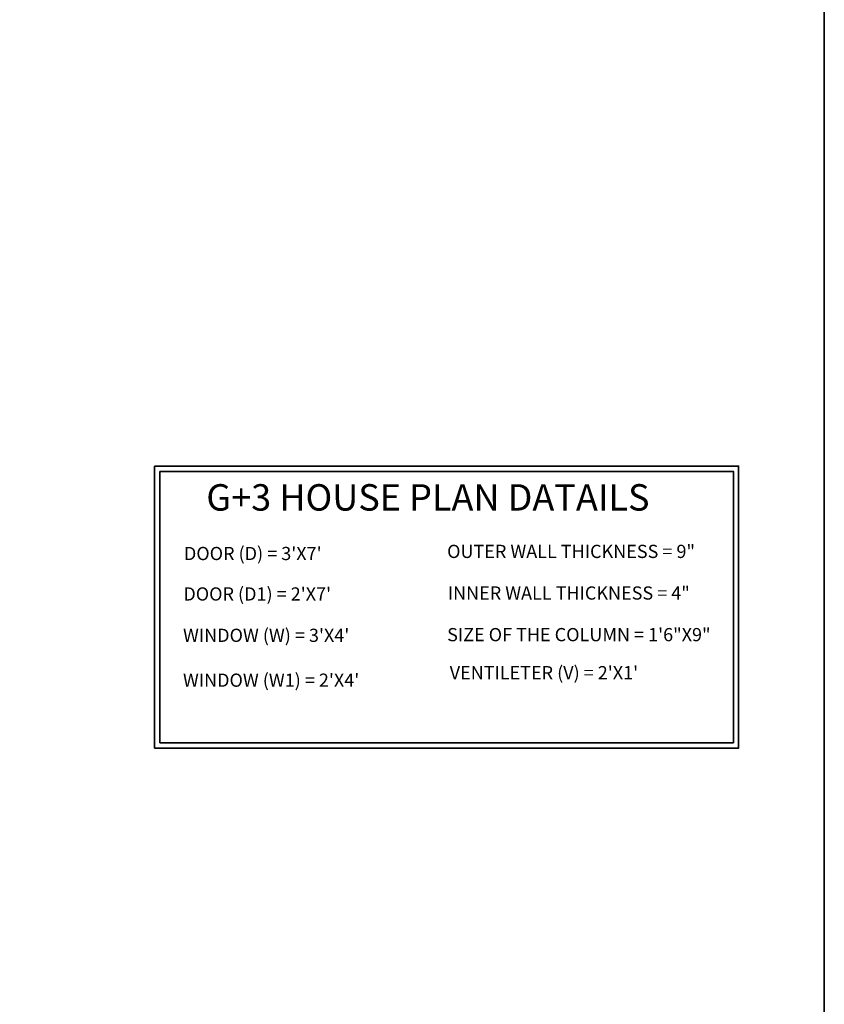
# Model space of a CAD drawing. Units: inches. Extents: x 2391 to 16591, y 7259 to 10239.
# Tile 21 of 27: x 3545 to 4154, y 8500 to 9245. Entities that reach past the tile are written whole.
import ezdxf

# ---------------------------------------------------------------- set-up
doc = ezdxf.new("R2010")
doc.units = ezdxf.units.IN
for name, color, linetype, lineweight in [('A-ANNO-TEXT', 4, 'Continuous', 18), ('A-ANNO-TITL', 3, 'Continuous', 30), ('A-ANNO-TTLB', 7, 'Continuous', 35)]:
    doc.layers.add(name, color=color, linetype=linetype, lineweight=lineweight)
doc.styles.get("Standard").update_dxf_attribs({"font": 'arial.ttf'})

msp = doc.modelspace()

# ---------------------------------------------------------------- linework, layer by layer
at = {"layer": 'A-ANNO-TTLB'}
for points in [[(2391.28, 10239.38), (4154.2, 10239.38), (4154.2, 7258.54), (2391.28, 7258.54)], [(3647.57, 8907.13), (4089.39, 8907.13), (4089.39, 8693.74), (3647.57, 8693.74)], [(3651.57, 8903.13), (4085.39, 8903.13), (4085.39, 8697.74), (3651.57, 8697.74)]]:
    msp.add_lwpolyline(points, close=True, dxfattribs=at)

# ---------------------------------------------------------------- texts
at = {"layer": 'A-ANNO-TEXT', "char_height": 10, "attachment_point": 1}
for s, width, insert in [("DOOR (D) = 3'X7'", 625.3197, (3669.71, 8846.01)), ('OUTER WALL THICKNESS = 9"', 390.9598, (3868.85, 8847.6)), ("DOOR (D1) = 2'X7'", 206.0633, (3669.3, 8815.4)), ('INNER WALL THICKNESS = 4"', 400.7416, (3869.32, 8816.11)), ("WINDOW (W) = 3'X4'", 352.4251, (3669.04, 8784.1)), ('SIZE OF THE COLUMN = 1\'6"X9"', 450.162, (3868.86, 8784.61)), ("VENTILETER (V) = 2'X1'", 248.9316, (3870.79, 8755.82)), ("WINDOW (W1) = 2'X4'", 250.7552, (3668.99, 8750.15))]:
    msp.add_mtext_dynamic_manual_height_columns(s, width=width, gutter_width=12.5, heights=[0], dxfattribs=dict(at, insert=insert))
at = {"layer": 'A-ANNO-TITL', "insert": (3686.66, 8893.47), "char_height": 20, "attachment_point": 1}
msp.add_mtext_dynamic_manual_height_columns('G+3 HOUSE PLAN DATAILS', width=378.5564, gutter_width=12.5, heights=[0], dxfattribs=at)

doc.saveas('drawing.dxf')
